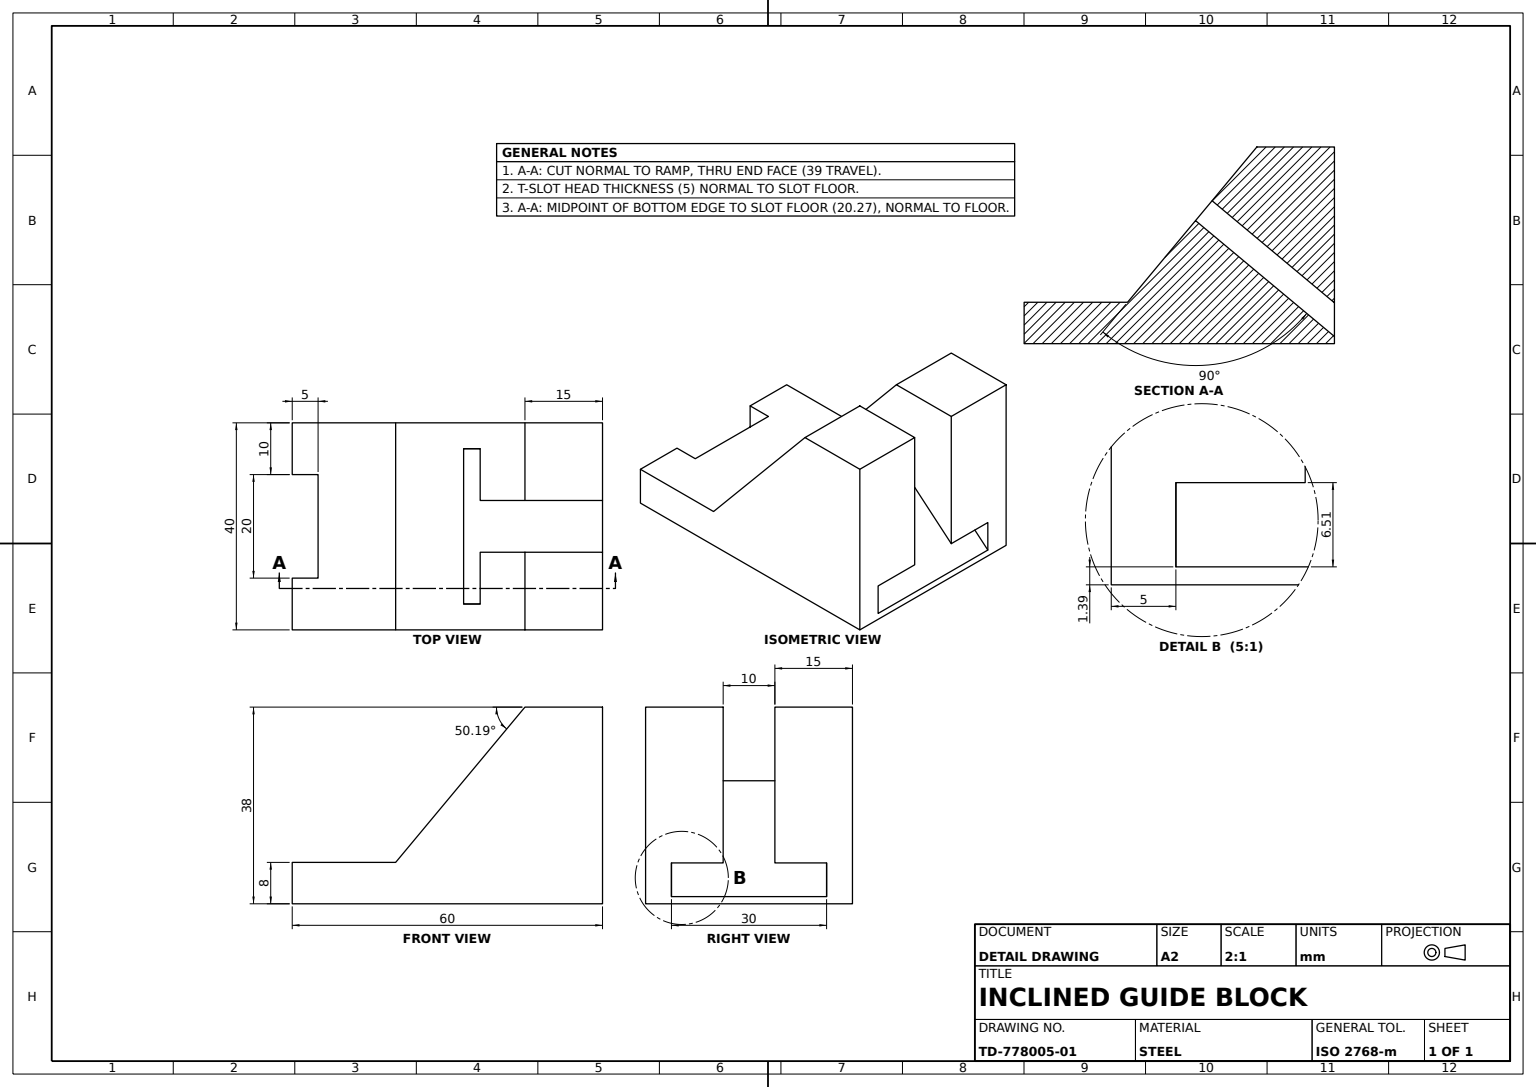
SolidWorks part; units mm, degrees
material "Plain Carbon Steel"
ref_plane "Front Plane" through (0, 0, 0) normal (0, 0, 1) x (1, 0, 0)
ref_plane "Top Plane" through (0, 0, 0) normal (0, 1, 0) x (1, 0, 0)
ref_plane "Right Plane" through (0, 0, 0) normal (1, 0, 0) x (0, 0, -1)
sketch "Base Plate Sketch" plane through (0, 0, 0) normal (0, 1, 0) x (1, 0, 0)
  line L1 (20, -30) -> (-20, -30)
  line L2 (20, -30) -> (20, 30)
  line L3 (20, 30) -> (-20, 30)
  line L4 (-20, -30) -> (-20, 30)
  line L5 (20, -30) -> (-20, 30) construction
  line L6 (20, 30) -> (-20, -30) construction
  point P0 (0, 0)
  dimension "D1" = 60
  dimension "D2" = 40
extrude "Base Plate 60x40x8" add sketch "Base Plate Sketch" along normal blind 8
sketch "Base Notch Sketch" plane through (0, 8, 0) normal (0, 1, 0) x (1, 0, 0)
  line L0 (-10, -30) -> (10, -30)
  line L2 (10, -30) -> (10, -25)
  line L3 (-10, -30) -> (-10, -25)
  line L4 (-10, -25) -> (10, -25)
  dimension "D1" = 20
  dimension "D4" = 30
  dimension "D2" = 5
  dimension "D3" = 10
extrude "Base Notch 20x5" cut sketch "Base Notch Sketch" against normal blind 20
sketch "Upright Block Sketch" plane through (20, 0, 0) normal (1, 0, 0) x (0, 0, -1)
  line L0 (30, 8) -> (-10, 8)
  line L1 (-30, 8) -> (30, 8) construction
  line L2 (30, 8) -> (30, 38)
  line L3 (30, 38) -> (-10, 38)
  line L4 (-10, 38) -> (-10, 8)
  dimension "D1" = 40
  dimension "D2" = 30
extrude "Upright Block 40x30x40" add sketch "Upright Block Sketch" against normal blind 40
sketch "Slope Cut Sketch" plane through (20, 0, 0) normal (1, 0, 0) x (0, 0, -1)
  line L0 (15, 38) -> (-10, 38)
  line L1 (30, 38) -> (-10, 38) construction
  line L2 (-10, 38) -> (-10, 8)
  line L4 (15, 38) -> (-10, 8)
  dimension "D1" = 15
extrude "Sloped Face Cut" cut sketch "Slope Cut Sketch" against normal blind 40
ref_plane "Plane2" through (0, 8.1967, 9.8361) normal (0, 0.6402, 0.7682) x (1, 0, 0)
sketch "Top Slot Sketch" plane through (0, 8.1967, 9.8361) normal (0, 0.6402, 0.7682) x (1, 0, 0)
  line L0 (-5, 25.2727) -> (-15, 25.2727)
  line L2 (-5, 38.7952) -> (-5, 25.2727)
  line L3 (5, 38.7952) -> (5, 25.2727)
  line L4 (-15, 25.2727) -> (-15, 20.2727)
  line L5 (-15, 20.2727) -> (15, 20.2727)
  line L6 (15, 20.2727) -> (15, 25.2727)
  line L7 (15, 25.2727) -> (5, 25.2727)
  line L8 (-20, 38.7952) -> (20, 38.7952) construction
  line L9 (-5, 38.7952) -> (5, 38.7952)
  dimension "D1" = 30
  dimension "D2" = 5
  dimension "D3" = 5
  dimension "D4" = 10
  dimension "D5" = 15
  dimension "D6" = 20.2727
extrude "Top Slot Cut" cut sketch "Top Slot Sketch" against normal blind 39
sketch "Angled Slot Sketch" plane through (0, 38, 0) normal (0, 1, 0) x (1, 0, 0)
  line L0 (5, 15) -> (5, 30)
  line L1 (-20, 30) -> (20, 30) construction
  line L2 (-5, 15) -> (-5, 30)
  line L3 (-5, 15) -> (5, 15)
  line L4 (-5, 30) -> (5, 30)
extrude "Angled Slot Through Sloped Face" cut sketch "Angled Slot Sketch" against normal up to next
